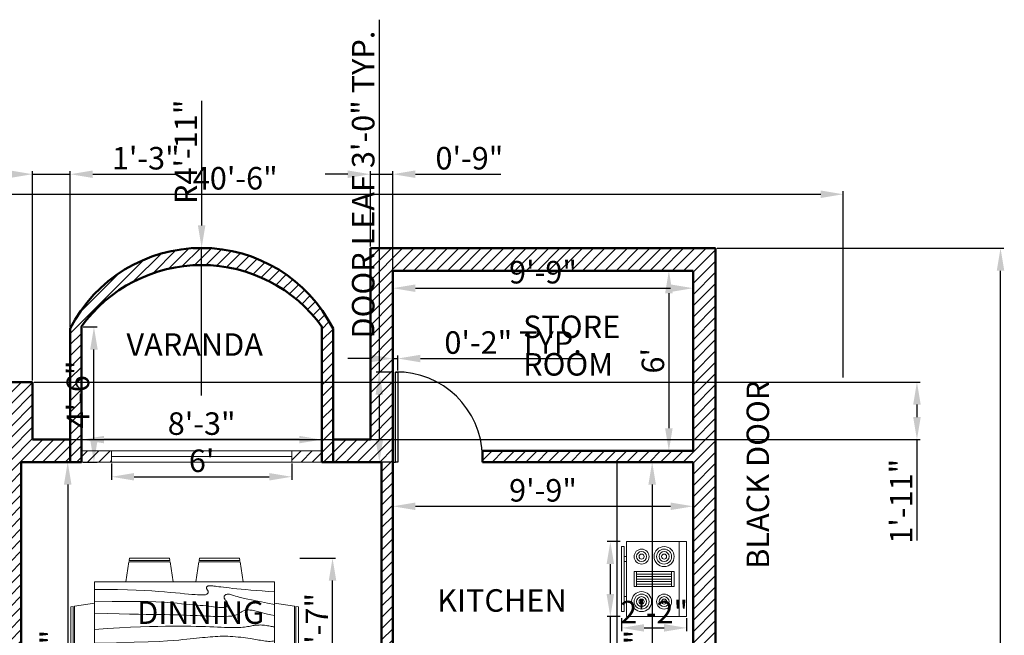
# Model space of a CAD drawing. Units: inches. Extents: x 5928 to 6612, y 5674 to 6320.
# Tile 5 of 5: x 6219 to 6612, y 6074 to 6320. Entities that reach past the tile are written whole.
import ezdxf

# ---------------------------------------------------------------- set-up
doc = ezdxf.new("R2010")
doc.units = ezdxf.units.IN
for name, color, linetype, lineweight in [('A-ANNO-DIMS', 2, 'Continuous', 18), ('A-ANNO-TEXT', 7, 'Continuous', 25), ('A-AREA-IDEN', 7, 'Continuous', 25), ('A-DOOR', 3, 'Continuous', 25), ('A-EQPM', 9, 'Continuous', 18), ('A-FLOR-CASE', 8, 'Continuous', 25), ('A-FURN', 8, 'Continuous', 18), ('A-GLAZ', 4, 'Continuous', 18), ('A-WALL', 7, 'Continuous', 50), ('A-WALL-PATT', 252, 'Continuous', 13)]:
    doc.layers.add(name, color=color, linetype=linetype, lineweight=lineweight)
doc.styles.get("Standard").update_dxf_attribs({"font": 'arial.ttf'})
doc.dimstyles.new('ISO-25', dxfattribs={"dimtxt": 9, "dimasz": 9, "dimexe": 1.25, "dimexo": 0.625, "dimtad": 1, "dimdec": 1, "dimrnd": 9, "dimlunit": 3, "dimtxsty": 'Standard', "dimcen": 2.5, "dimadec": 0, "dimazin": 0, "dimtfac": 1, "dimtdec": 1, "dimtmove": 0, "dimatfit": 3, "dimfxl": 1, "dimarcsym": 0})

# ---------------------------------------------------------------- blocks, each defined once
blk = doc.blocks.new('Dining Set - 36 x 72 in.')
for p, q in [((-22.2343, 26.00059), (-23.4847, 17.99762)), ((-22.2304, 26), (-5.7608, 26)), ((-22, 27.5), (-22.1562, 26.50042)), ((-5.8416, 26.5), (-22.1534, 26.5)), ((-22, 27.5), (-6, 27.5)), ((-5.8437, 26.49966), (-6, 27.5)), ((-4.5152, 17.99762), (-5.7655, 25.99926)), ((5.7657, 26.00059), (4.5153, 17.99762)), ((5.7696, 26), (22.2392, 26)), ((6, 27.5), (5.8438, 26.50042)), ((22.1584, 26.5), (5.8466, 26.5)), ((6, 27.5), (22, 27.5)), ((22.1563, 26.49966), (22, 27.5)), ((23.4848, 17.99762), (22.2345, 25.99926)), ((36, 18), (-36, 18)), ((-36, 18), (-36, -18)), ((36, -18), (36, 18)), ((-45.5, 8), (-44.5004, 8.15617)), ((-45.5, 8), (-45.5, -8)), ((-44.5, -8.15843), (-44.5, 8.15338)), ((-44.0006, 8.23428), (-35.9976, 9.48474)), ((-44, 8.23041), (-44, -8.23915)), ((44.0006, 8.23428), (35.9976, 9.48474)), ((44, 8.23041), (44, -8.23915)), ((44.5, -8.15843), (44.5, 8.15338)), ((45.5, 8), (44.5005, 8.15617)), ((45.5, 8), (45.5, -8)), ((-44.4997, -8.15631), (-45.5, -8)), ((-35.9976, -9.48476), (-43.9993, -8.2345)), ((35.9976, -9.48476), (43.9993, -8.2345)), ((44.4997, -8.15631), (45.5, -8)), ((-36, -18), (36, -18)), ((-22.2343, -26.0006), (-23.4847, -17.99762)), ((-4.5152, -17.99762), (-5.7655, -25.99928)), ((5.7657, -26.0006), (4.5153, -17.99762)), ((23.4848, -17.99762), (22.2345, -25.99928)), ((-22.2304, -26), (-5.7608, -26)), ((-22, -27.5), (-22.1562, -26.50044)), ((-5.8416, -26.5), (-22.1534, -26.5)), ((-22, -27.5), (-6, -27.5)), ((-5.8437, -26.49967), (-6, -27.5)), ((5.7696, -26), (22.2392, -26)), ((6, -27.5), (5.8438, -26.50044)), ((22.1584, -26.5), (5.8466, -26.5)), ((6, -27.5), (22, -27.5)), ((22.1563, -26.49967), (22, -27.5))]:
    blk.add_line(p, q)
for points in [[(-36, 15), (-31.1772, 14.97754), (-26.8079, 14.91406), (-22.8538, 14.81543), (-19.276, 14.6875), (-16.0362, 14.53613), (-13.0957, 14.36718), (-10.4159, 14.18652), (-7.9583, 14), (-5.6904, 13.81315), (-3.6035, 13.63021), (-1.6954, 13.45508), (0.0365, 13.29166), (1.5945, 13.14388), (2.9811, 13.01562), (4.1988, 12.9108), (5.25, 12.83333), (6.1393, 12.78613), (6.8802, 12.76823), (7.4883, 12.77767), (7.9792, 12.8125), (8.3685, 12.87077), (8.6719, 12.95052), (8.9049, 13.0498), (9.0833, 13.16666), (9.2205, 13.29899), (9.3216, 13.44401), (9.3895, 13.59879), (9.4271, 13.76041), (9.4373, 13.92594), (9.4232, 14.09245), (9.3875, 14.257), (9.3333, 14.41666), (9.2638, 14.56917), (9.1836, 14.71484), (9.0975, 14.85465), (9.0104, 14.98958), (8.9272, 15.1206), (8.8529, 15.2487), (8.7922, 15.37483), (8.75, 15.5), (8.7305, 15.62467), (8.7344, 15.74739), (8.7617, 15.86621), (8.8125, 15.97916), (8.8867, 16.08431), (8.9844, 16.17968), (9.1055, 16.26334), (9.25, 16.33333), (9.4189, 16.38802), (9.6172, 16.42708), (9.8506, 16.45052), (10.125, 16.45833), (10.4463, 16.45052), (10.8203, 16.42708), (11.2529, 16.38802), (11.75, 16.33333), (12.3184, 16.26318), (12.9694, 16.17838), (13.7151, 16.07991), (14.5677, 15.96875), (15.5395, 15.84586), (16.6426, 15.71224), (17.8893, 15.56884), (19.2917, 15.41666), (20.859, 15.25667), (22.5879, 15.08984), (24.4721, 14.91715), (26.5052, 14.73958), (28.6809, 14.5581), (30.9929, 14.3737), (33.4347, 14.18733), (36, 14)], [(-36, 10), (-28.9766, 10.14274), (-23.1725, 10.20442), (-18.4241, 10.19775), (-14.5677, 10.13541), (-11.4399, 10.03011), (-8.877, 9.89453), (-6.7154, 9.74137), (-4.7917, 9.58333), (-2.9698, 9.43082), (-1.2246, 9.28515), (0.4415, 9.14534), (2.026, 9.01041), (3.5266, 8.87939), (4.9408, 8.7513), (6.266, 8.62516), (7.5, 8.5), (8.6411, 8.37549), (9.6914, 8.2539), (10.6538, 8.13818), (11.5312, 8.03125), (12.3267, 7.93603), (13.043, 7.85547), (13.6831, 7.79248), (14.25, 7.75), (14.7471, 7.7303), (15.1797, 7.73307), (15.5537, 7.75732), (15.875, 7.80208), (16.1494, 7.86637), (16.3828, 7.94922), (16.5811, 8.04964), (16.75, 8.16666), (16.8944, 8.29915), (17.0143, 8.44531), (17.1089, 8.60319), (17.1771, 8.77083), (17.218, 8.94629), (17.2305, 9.1276), (17.2137, 9.31282), (17.1667, 9.5), (17.0895, 9.6875), (16.987, 9.875), (16.8649, 10.0625), (16.7292, 10.25), (16.5856, 10.4375), (16.4401, 10.625), (16.2985, 10.8125), (16.1667, 11), (16.05, 11.18733), (15.9518, 11.3737), (15.8752, 11.5581), (15.8229, 11.73958), (15.798, 11.91715), (15.8034, 12.08984), (15.842, 12.25667), (15.9167, 12.41666), (16.0295, 12.56836), (16.1784, 12.70833), (16.3605, 12.83268), (16.5729, 12.9375), (16.8127, 13.01888), (17.0768, 13.07291), (17.3625, 13.0957), (17.6667, 13.08333), (17.9894, 13.03312), (18.3418, 12.94726), (18.7382, 12.82918), (19.1927, 12.68229), (19.7195, 12.51001), (20.3327, 12.31575), (21.0465, 12.10294), (21.875, 11.875), (22.8357, 11.63354), (23.959, 11.37304), (25.2786, 11.08618), (26.8282, 10.76562), (28.6414, 10.40405), (30.752, 9.99414), (33.1936, 9.52856), (36, 9)], [(-36, 5.5), (-30.7157, 5.3348), (-26.069, 5.20963), (-21.9946, 5.11767), (-18.4271, 5.05208), (-15.3009, 5.00602), (-12.5508, 4.97265), (-10.1112, 4.94515), (-7.9167, 4.91666), (-5.909, 4.88167), (-4.0586, 4.83984), (-2.3429, 4.79215), (-0.7396, 4.73958), (0.7739, 4.6831), (2.22, 4.6237), (3.6213, 4.56233), (5, 4.5), (6.373, 4.43782), (7.7344, 4.3776), (9.0723, 4.32129), (10.375, 4.27083), (11.6309, 4.22819), (12.8281, 4.19531), (13.9551, 4.17415), (15, 4.16666), (15.954, 4.17448), (16.819, 4.19791), (17.6001, 4.23698), (18.3021, 4.29166), (18.9299, 4.36198), (19.4883, 4.44791), (19.9823, 4.54948), (20.4167, 4.66666), (20.7969, 4.79899), (21.1302, 4.94401), (21.4245, 5.09879), (21.6875, 5.26041), (21.9271, 5.42594), (22.1511, 5.59245), (22.3672, 5.757), (22.5834, 5.91666), (22.8065, 6.06868), (23.0404, 6.21093), (23.2879, 6.34147), (23.5521, 6.45833), (23.8358, 6.55957), (24.142, 6.64323), (24.4735, 6.70735), (24.8334, 6.75), (25.2235, 6.76969), (25.642, 6.76692), (26.0858, 6.74267), (26.5521, 6.69791), (27.0379, 6.63362), (27.5404, 6.55078), (28.0565, 6.45036), (28.5834, 6.33333), (29.1242, 6.19987), (29.7071, 6.04687), (30.3661, 5.87044), (31.1354, 5.66666), (32.0493, 5.43164), (33.142, 5.16146), (34.4475, 4.85221), (36, 4.5)], [(-36, -1), (-30.7915, -0.6591), (-26.0195, -0.38216), (-21.6519, -0.16284), (-17.6563, 0.00521), (-14.0005, 0.12833), (-10.6523, 0.21289), (-7.5796, 0.26522), (-4.75, 0.29166), (-2.134, 0.29793), (0.2878, 0.28711), (2.5317, 0.26163), (4.6146, 0.22396), (6.5529, 0.17651), (8.3633, 0.12174), (10.0623, 0.06209), (11.6667, 0), (13.1899, -0.06201), (14.6341, -0.1211), (15.9982, -0.17432), (17.2813, -0.21875), (18.4823, -0.25147), (19.6003, -0.26953), (20.6343, -0.27002), (21.5834, -0.25), (22.4481, -0.20768), (23.2357, -0.14584), (23.9549, -0.06836), (24.6146, 0.02083), (25.2235, 0.11784), (25.7904, 0.21875), (26.3241, 0.31966), (26.8334, 0.41666), (27.3265, 0.50618), (27.8099, 0.58593), (28.2894, 0.65397), (28.7709, 0.70833), (29.2601, 0.74707), (29.763, 0.76823), (30.2855, 0.76985), (30.8334, 0.75), (31.4088, 0.70784), (31.9994, 0.64713), (32.589, 0.57275), (33.1615, 0.48958), (33.7008, 0.4025), (34.1908, 0.3164), (34.6153, 0.23616), (34.9584, 0.16666), (35.2099, 0.11165), (35.3848, 0.07031), (35.504, 0.04069), (35.5886, 0.02083), (35.6594, 0.00879), (35.7377, 0.0026), (35.8442, 0.00032), (36, 0)], [(-36, -6.5), (-27.1843, -6.31267), (-20.084, -6.1263), (-14.469, -5.9419), (-10.1094, -5.76042), (-6.7752, -5.58285), (-4.2363, -5.41016), (-2.2629, -5.24333), (-0.625, -5.08334), (0.8708, -4.93099), (2.2715, -4.78646), (3.5872, -4.64974), (4.8281, -4.52084), (6.0046, -4.39974), (7.127, -4.28646), (8.2053, -4.18099), (9.25, -4.08334), (10.2705, -3.99382), (11.2734, -3.91407), (12.2647, -3.84603), (13.25, -3.79167), (14.2354, -3.75293), (15.2266, -3.73177), (16.2295, -3.73015), (17.25, -3.75), (18.2912, -3.79248), (19.3451, -3.85547), (20.4009, -3.93604), (21.4479, -4.03125), (22.4754, -4.13819), (23.4727, -4.25391), (24.4289, -4.37549), (25.3334, -4.5), (26.1785, -4.62492), (26.9694, -4.74935), (27.7145, -4.87281), (28.4219, -4.99479), (29.1, -5.11483), (29.7572, -5.23242), (30.4016, -5.34709), (31.0417, -5.45834), (31.6837, -5.56437), (32.3262, -5.65821), (32.9658, -5.73153), (33.599, -5.77604), (34.2224, -5.78345), (34.8327, -5.74545), (35.4264, -5.65373), (36, -5.5)], [(-36, -10), (-26.4022, -9.81299), (-18.4675, -9.62891), (-11.9839, -9.45069), (-6.7396, -9.28125), (-2.5226, -9.12354), (0.8789, -8.98047), (3.6769, -8.85498), (6.0833, -8.75), (8.2767, -8.66765), (10.3021, -8.60677), (12.1712, -8.56543), (13.8958, -8.54167), (15.4876, -8.53353), (16.9583, -8.53907), (18.3197, -8.55632), (19.5834, -8.58334), (20.7616, -8.61841), (21.8685, -8.66081), (22.9188, -8.71004), (23.9271, -8.76563), (24.9081, -8.82707), (25.8763, -8.89388), (26.8465, -8.96558), (27.8334, -9.04167), (28.8474, -9.12118), (29.8828, -9.20117), (30.93, -9.27824), (31.9792, -9.34896), (33.0205, -9.40991), (34.0443, -9.45768), (35.0407, -9.48885), (36, -9.5)], [(-36, -14.5), (-30.0881, -14.33513), (-25.0332, -14.21224), (-20.7312, -14.12647), (-17.0781, -14.07292), (-13.97, -14.04671), (-11.3027, -14.04297), (-8.9724, -14.05681), (-6.875, -14.08334), (-4.9224, -14.11833), (-3.0905, -14.16016), (-1.3709, -14.20785), (0.2448, -14.26042), (1.7647, -14.3169), (3.1973, -14.3763), (4.5507, -14.43767), (5.8333, -14.5), (7.0554, -14.5621), (8.235, -14.62175), (9.3922, -14.67652), (10.5469, -14.72396), (11.7192, -14.76164), (12.929, -14.78711), (14.1965, -14.79794), (15.5417, -14.79167), (16.9933, -14.76424), (18.6152, -14.70508), (20.4804, -14.60197), (22.6615, -14.44271), (25.2312, -14.21509), (28.2624, -13.9069), (31.8277, -13.50594), (36, -13)]]:
    blk.add_lwpolyline(points)
blk = doc.blocks.new('Range-Oven - 30 in top')
for p, q in [((0, -3), (30, -3)), ((12, -6), (18, -6)), ((13, -20), (13, -6)), ((14, -6), (14, -20)), ((15, -20), (15, -6)), ((16, -6), (16, -20)), ((17, -20), (17, -6)), ((18, -20), (12, -20)), ((6, -24), (6, -25)), ((8, -25), (8, -24)), ((22, -25), (22, -24)), ((24, -24), (24, -25))]:
    blk.add_line(p, q)
for points in [[(0, -24), (0, 0), (30, 0), (30, -24)], [(12, -21), (12, -5), (18, -5), (18, -21)], [(2, -26), (2, -25), (28, -25), (28, -26)]]:
    blk.add_lwpolyline(points, close=True)
for centre, radius in [((6, -9), 4), ((6, -9), 3), ((6, -9), 2), ((24, -9), 3), ((24, -9), 2), ((6, -9), 1), ((24, -9), 1), ((6, -18), 3), ((24, -18), 4), ((24, -18), 3), ((6, -18), 2), ((6, -18), 1), ((24, -18), 2), ((24, -18), 1)]:
    blk.add_circle(centre, radius)
blk = doc.blocks.new('*D23')
at = {"layer": 'A-ANNO-DIMS', "color": 0, "lineweight": -2, "transparency": 16777216}
for p, q in [((6220.15, 6142.76), (6239.34, 6142.76)), ((6238.09, 6133.76), (6238.09, 5983.76)), ((6220.15, 5974.76), (6239.34, 5974.76))]:
    blk.add_line(p, q, dxfattribs=at)
at = {"layer": 'A-ANNO-DIMS', "color": 0, "transparency": 16777216}
for points in [[(6236.59, 6133.76), (6239.59, 6133.76), (6238.09, 6142.76)], [(6236.59, 5983.76), (6239.59, 5983.76), (6238.09, 5974.76)]]:
    blk.add_solid(points, dxfattribs=at)
at = {"layer": 'Defpoints', "color": 0, "transparency": 16777216}
for p in [(6219.53, 6142.76), (6219.53, 5974.76), (6238.09, 5974.76)]:
    blk.add_point(p, dxfattribs=at)
at = {"layer": 'A-ANNO-DIMS', "color": 0, "transparency": 16777216, "insert": (6232.87, 6058.76), "char_height": 9, "attachment_point": 5, "rotation": 90}
blk.add_mtext('14\'-3"', dxfattribs=at)
blk = doc.blocks.new('*D27')
at = {"layer": 'A-ANNO-DIMS', "color": 0, "lineweight": -2, "transparency": 16777216}
for p, q in [((6243.61, 6147.89), (6243.61, 6153)), ((6330.61, 6151.75), (6252.61, 6151.75)), ((6339.61, 6147.89), (6339.61, 6153))]:
    blk.add_line(p, q, dxfattribs=at)
at = {"layer": 'A-ANNO-DIMS', "color": 0, "transparency": 16777216}
for points in [[(6252.61, 6153.25), (6252.61, 6150.25), (6243.61, 6151.75)], [(6330.61, 6153.25), (6330.61, 6150.25), (6339.61, 6151.75)]]:
    blk.add_solid(points, dxfattribs=at)
at = {"layer": 'Defpoints', "color": 0, "transparency": 16777216}
for p in [(6243.61, 6151.75), (6243.61, 6147.26), (6339.61, 6147.26)]:
    blk.add_point(p, dxfattribs=at)
at = {"layer": 'A-ANNO-DIMS', "color": 0, "transparency": 16777216, "insert": (6291.61, 6156.98), "char_height": 9, "attachment_point": 5}
blk.add_mtext('8\'-3"', dxfattribs=at)
blk = doc.blocks.new('*D28')
at = {"layer": 'A-ANNO-DIMS', "color": 0, "lineweight": -2, "transparency": 16777216}
for p, q in [((6255.61, 6142.14), (6255.61, 6135.65)), ((6327.61, 6142.14), (6327.61, 6135.65)), ((6264.61, 6136.9), (6318.61, 6136.9))]:
    blk.add_line(p, q, dxfattribs=at)
at = {"layer": 'A-ANNO-DIMS', "color": 0, "transparency": 16777216}
for points in [[(6264.61, 6138.4), (6264.61, 6135.4), (6255.61, 6136.9)], [(6318.61, 6138.4), (6318.61, 6135.4), (6327.61, 6136.9)]]:
    blk.add_solid(points, dxfattribs=at)
at = {"layer": 'Defpoints', "color": 0, "transparency": 16777216}
for p in [(6255.61, 6142.76), (6327.61, 6142.76), (6327.61, 6136.9)]:
    blk.add_point(p, dxfattribs=at)
at = {"layer": 'A-ANNO-DIMS', "color": 0, "transparency": 16777216, "insert": (6291.61, 6142.12), "char_height": 9, "attachment_point": 5}
blk.add_mtext("6'", dxfattribs=at)
blk = doc.blocks.new('*D29')
at = {"layer": 'A-ANNO-DIMS', "color": 0, "lineweight": -2, "transparency": 16777216}
for p, q in [((6244.23, 6196.76), (6249.81, 6196.76)), ((6248.56, 6151.76), (6248.56, 6187.76)), ((6244.23, 6142.76), (6249.81, 6142.76))]:
    blk.add_line(p, q, dxfattribs=at)
at = {"layer": 'A-ANNO-DIMS', "color": 0, "transparency": 16777216}
for points in [[(6247.06, 6187.76), (6250.06, 6187.76), (6248.56, 6196.76)], [(6247.06, 6151.76), (6250.06, 6151.76), (6248.56, 6142.76)]]:
    blk.add_solid(points, dxfattribs=at)
at = {"layer": 'Defpoints', "color": 0, "transparency": 16777216}
for p in [(6243.61, 6196.76), (6248.56, 6196.76), (6243.61, 6142.76)]:
    blk.add_point(p, dxfattribs=at)
at = {"layer": 'A-ANNO-DIMS', "color": 0, "transparency": 16777216, "insert": (6243.34, 6169.76), "char_height": 9, "attachment_point": 5, "rotation": 90}
blk.add_mtext('4\'-6"', dxfattribs=at)
blk = doc.blocks.new('*D30')
at = {"layer": 'A-ANNO-DIMS', "color": 0, "lineweight": -2, "transparency": 16777216}
for p, q in [((6368.03, 6218.64), (6368.03, 6211.02)), ((6488.03, 6218.64), (6488.03, 6211.02)), ((6377.03, 6212.27), (6479.03, 6212.27))]:
    blk.add_line(p, q, dxfattribs=at)
at = {"layer": 'A-ANNO-DIMS', "color": 0, "transparency": 16777216}
for points in [[(6377.03, 6213.77), (6377.03, 6210.77), (6368.03, 6212.27)], [(6479.03, 6213.77), (6479.03, 6210.77), (6488.03, 6212.27)]]:
    blk.add_solid(points, dxfattribs=at)
at = {"layer": 'Defpoints', "color": 0, "transparency": 16777216}
for p in [(6368.03, 6219.26), (6488.03, 6219.26), (6488.03, 6212.27)]:
    blk.add_point(p, dxfattribs=at)
at = {"layer": 'A-ANNO-DIMS', "color": 0, "transparency": 16777216, "insert": (6428.03, 6217.49), "char_height": 9, "attachment_point": 5}
blk.add_mtext('9\'-9"', dxfattribs=at)
blk = doc.blocks.new('*D31')
at = {"layer": 'A-ANNO-DIMS', "color": 0, "lineweight": -2, "transparency": 16777216}
for p, q in [((6487.4, 6219.26), (6477.09, 6219.26)), ((6478.34, 6210.26), (6478.34, 6156.26)), ((6487.4, 6147.26), (6477.09, 6147.26))]:
    blk.add_line(p, q, dxfattribs=at)
at = {"layer": 'A-ANNO-DIMS', "color": 0, "transparency": 16777216}
for points in [[(6476.84, 6210.26), (6479.84, 6210.26), (6478.34, 6219.26)], [(6476.84, 6156.26), (6479.84, 6156.26), (6478.34, 6147.26)]]:
    blk.add_solid(points, dxfattribs=at)
at = {"layer": 'Defpoints', "color": 0, "transparency": 16777216}
for p in [(6488.03, 6219.26), (6478.34, 6147.26), (6488.03, 6147.26)]:
    blk.add_point(p, dxfattribs=at)
at = {"layer": 'A-ANNO-DIMS', "color": 0, "transparency": 16777216, "insert": (6473.12, 6183.26), "char_height": 9, "attachment_point": 5, "rotation": 90}
blk.add_mtext("6'", dxfattribs=at)
blk = doc.blocks.new('*D34')
at = {"layer": 'A-ANNO-DIMS', "color": 0, "lineweight": -2, "transparency": 16777216}
for p, q in [((6487.4, 6142.76), (6470.41, 6142.76)), ((6471.66, 6133.76), (6471.66, 5983.76)), ((6487.4, 5974.76), (6470.41, 5974.76))]:
    blk.add_line(p, q, dxfattribs=at)
at = {"layer": 'A-ANNO-DIMS', "color": 0, "transparency": 16777216}
for points in [[(6470.16, 6133.76), (6473.16, 6133.76), (6471.66, 6142.76)], [(6470.16, 5983.76), (6473.16, 5983.76), (6471.66, 5974.76)]]:
    blk.add_solid(points, dxfattribs=at)
at = {"layer": 'Defpoints', "color": 0, "transparency": 16777216}
for p in [(6488.03, 6142.76), (6471.66, 5974.76), (6488.03, 5974.76)]:
    blk.add_point(p, dxfattribs=at)
at = {"layer": 'A-ANNO-DIMS', "color": 0, "transparency": 16777216, "insert": (6466.44, 6058.76), "char_height": 9, "attachment_point": 5, "rotation": 90}
blk.add_mtext('14\'-3"', dxfattribs=at)
blk = doc.blocks.new('*D35')
at = {"layer": 'A-ANNO-DIMS', "color": 0, "lineweight": -2, "transparency": 16777216}
for p, q in [((6368.03, 6142.14), (6368.03, 6123.85)), ((6488.03, 6142.14), (6488.03, 6123.85)), ((6377.03, 6125.1), (6479.03, 6125.1))]:
    blk.add_line(p, q, dxfattribs=at)
at = {"layer": 'A-ANNO-DIMS', "color": 0, "transparency": 16777216}
for points in [[(6377.03, 6126.6), (6377.03, 6123.6), (6368.03, 6125.1)], [(6479.03, 6126.6), (6479.03, 6123.6), (6488.03, 6125.1)]]:
    blk.add_solid(points, dxfattribs=at)
at = {"layer": 'Defpoints', "color": 0, "transparency": 16777216}
for p in [(6368.03, 6142.76), (6488.03, 6142.76), (6488.03, 6125.1)]:
    blk.add_point(p, dxfattribs=at)
at = {"layer": 'A-ANNO-DIMS', "color": 0, "transparency": 16777216, "insert": (6428.03, 6130.32), "char_height": 9, "attachment_point": 5}
blk.add_mtext('9\'-9"', dxfattribs=at)
blk = doc.blocks.new('*D36')
at = {"layer": 'A-ANNO-DIMS', "color": 0, "lineweight": -2, "transparency": 16777216}
for p, q in [((6062.03, 6175.39), (6062.03, 6251.06)), ((6071.03, 6249.81), (6539.03, 6249.81)), ((6548.03, 6176.51), (6548.03, 6251.06))]:
    blk.add_line(p, q, dxfattribs=at)
at = {"layer": 'A-ANNO-DIMS', "color": 0, "transparency": 16777216}
for points in [[(6071.03, 6251.31), (6071.03, 6248.31), (6062.03, 6249.81)], [(6539.03, 6251.31), (6539.03, 6248.31), (6548.03, 6249.81)]]:
    blk.add_solid(points, dxfattribs=at)
at = {"layer": 'Defpoints', "color": 0, "transparency": 16777216}
for p in [(6548.03, 6249.81), (6062.03, 6174.76), (6548.03, 6175.89)]:
    blk.add_point(p, dxfattribs=at)
at = {"layer": 'A-ANNO-DIMS', "color": 0, "transparency": 16777216, "insert": (6305.03, 6255.03), "char_height": 9, "attachment_point": 5}
blk.add_mtext('40\'-6"', dxfattribs=at)
blk = doc.blocks.new('*D37')
at = {"layer": 'A-ANNO-DIMS', "color": 0, "lineweight": -2, "transparency": 16777216}
for p, q in [((6497.65, 6228.26), (6612.14, 6228.26)), ((6610.89, 5720.26), (6610.89, 6219.26)), ((6424.38, 5711.26), (6612.14, 5711.26))]:
    blk.add_line(p, q, dxfattribs=at)
at = {"layer": 'A-ANNO-DIMS', "color": 0, "transparency": 16777216}
for points in [[(6609.39, 6219.26), (6612.39, 6219.26), (6610.89, 6228.26)], [(6609.39, 5720.26), (6612.39, 5720.26), (6610.89, 5711.26)]]:
    blk.add_solid(points, dxfattribs=at)
at = {"layer": 'Defpoints', "color": 0, "transparency": 16777216}
for p in [(6497.03, 6228.26), (6610.89, 6228.26), (6423.76, 5711.26)]:
    blk.add_point(p, dxfattribs=at)
at = {"layer": 'A-ANNO-DIMS', "color": 0, "transparency": 16777216, "insert": (6605.67, 5969.76), "char_height": 9, "attachment_point": 5, "rotation": 90}
blk.add_mtext('42\'-9"', dxfattribs=at)
blk = doc.blocks.new('DOOR-LEAF-36IN')
for p, q in [((0, 0), (0, 36)), ((0, 36), (1, 36)), ((1, 36), (1, 0)), ((-1, 0), (0, 0)), ((1, 0), (0, 0))]:
    blk.add_line(p, q)
blk = doc.blocks.new('*D58')
at = {"layer": 'A-ANNO-DIMS', "color": 0, "lineweight": -2, "transparency": 16777216}
for p, q in [((6362.63, 6178.76), (6362.63, 6319.58)), ((6367.4, 6178.76), (6361.38, 6178.76)), ((6362.63, 6151.76), (6362.63, 6169.76)), ((6367.4, 6142.76), (6361.38, 6142.76))]:
    blk.add_line(p, q, dxfattribs=at)
at = {"layer": 'A-ANNO-DIMS', "color": 0, "transparency": 16777216}
for points in [[(6361.13, 6169.76), (6364.13, 6169.76), (6362.63, 6178.76)], [(6361.13, 6151.76), (6364.13, 6151.76), (6362.63, 6142.76)]]:
    blk.add_solid(points, dxfattribs=at)
at = {"layer": 'Defpoints', "color": 0, "transparency": 16777216}
for p in [(6362.63, 6178.76), (6368.03, 6178.76), (6368.03, 6142.76)]:
    blk.add_point(p, dxfattribs=at)
at = {"layer": 'A-ANNO-DIMS', "color": 0, "transparency": 16777216, "insert": (6357.34, 6253.67), "char_height": 9, "attachment_point": 5, "rotation": 90}
blk.add_mtext('DOOR LEAF 3\'-0" TYP.', dxfattribs=at)
blk = doc.blocks.new('*D59')
at = {"layer": 'A-ANNO-DIMS', "color": 0, "lineweight": -2, "transparency": 16777216}
for p, q in [((6359.03, 6184.16), (6350.03, 6184.16)), ((6368.03, 6179.39), (6368.03, 6185.41)), ((6368.03, 6184.16), (6370.03, 6184.16)), ((6370.03, 6179.39), (6370.03, 6185.41)), ((6379.03, 6184.16), (6444.14, 6184.16))]:
    blk.add_line(p, q, dxfattribs=at)
at = {"layer": 'A-ANNO-DIMS', "color": 0, "transparency": 16777216}
for points in [[(6359.03, 6185.66), (6359.03, 6182.66), (6368.03, 6184.16)], [(6379.03, 6185.66), (6379.03, 6182.66), (6370.03, 6184.16)]]:
    blk.add_solid(points, dxfattribs=at)
at = {"layer": 'Defpoints', "color": 0, "transparency": 16777216}
for p in [(6370.03, 6184.16), (6368.03, 6178.76), (6370.03, 6178.76)]:
    blk.add_point(p, dxfattribs=at)
at = {"layer": 'A-ANNO-DIMS', "color": 0, "transparency": 16777216, "insert": (6416.08, 6189.38), "char_height": 9, "attachment_point": 5}
blk.add_mtext('0\'-2" TYP.', dxfattribs=at)
blk = doc.blocks.new('*D65')
at = {"layer": 'A-ANNO-DIMS', "color": 0, "lineweight": -2, "transparency": 16777216}
for p, q in [((6330.9, 6104.39), (6345.17, 6104.39)), ((6343.92, 6058.39), (6343.92, 6095.39)), ((6330.9, 6049.39), (6345.17, 6049.39))]:
    blk.add_line(p, q, dxfattribs=at)
at = {"layer": 'A-ANNO-DIMS', "color": 0, "transparency": 16777216}
for points in [[(6342.42, 6095.39), (6345.42, 6095.39), (6343.92, 6104.39)], [(6342.42, 6058.39), (6345.42, 6058.39), (6343.92, 6049.39)]]:
    blk.add_solid(points, dxfattribs=at)
at = {"layer": 'Defpoints', "color": 0, "transparency": 16777216}
for p in [(6330.27, 6104.39), (6343.92, 6104.39), (6330.27, 6049.39)]:
    blk.add_point(p, dxfattribs=at)
at = {"layer": 'A-ANNO-DIMS', "color": 0, "transparency": 16777216, "insert": (6338.8, 6076.89), "char_height": 9, "attachment_point": 5, "rotation": 90}
blk.add_mtext('4\'-7"', dxfattribs=at)
blk = doc.blocks.new('*D66')
at = {"layer": 'A-ANNO-DIMS', "color": 0, "lineweight": -2, "transparency": 16777216}
for p, q in [((6458.82, 6111), (6453.69, 6111)), ((6454.94, 6102), (6454.94, 6090)), ((6458.82, 6081), (6453.69, 6081)), ((6454.94, 6081), (6454.94, 5999.09))]:
    blk.add_line(p, q, dxfattribs=at)
at = {"layer": 'A-ANNO-DIMS', "color": 0, "transparency": 16777216}
for points in [[(6453.44, 6102), (6456.44, 6102), (6454.94, 6111)], [(6453.44, 6090), (6456.44, 6090), (6454.94, 6081)]]:
    blk.add_solid(points, dxfattribs=at)
at = {"layer": 'Defpoints', "color": 0, "transparency": 16777216}
for p in [(6459.44, 6111), (6454.94, 6081), (6459.44, 6081)]:
    blk.add_point(p, dxfattribs=at)
at = {"layer": 'A-ANNO-DIMS', "color": 0, "transparency": 16777216, "insert": (6449.67, 6035.54), "char_height": 9, "attachment_point": 5, "rotation": 90}
blk.add_mtext('RANGE 2\'-6"', dxfattribs=at)
blk = doc.blocks.new('*D67')
at = {"layer": 'A-ANNO-DIMS', "color": 0, "lineweight": -2, "transparency": 16777216}
for p, q in [((6459.44, 6080.37), (6459.44, 6075.25)), ((6485.44, 6080.37), (6485.44, 6075.25)), ((6468.44, 6076.5), (6476.44, 6076.5))]:
    blk.add_line(p, q, dxfattribs=at)
at = {"layer": 'A-ANNO-DIMS', "color": 0, "transparency": 16777216}
for points in [[(6468.44, 6078), (6468.44, 6075), (6459.44, 6076.5)], [(6476.44, 6078), (6476.44, 6075), (6485.44, 6076.5)]]:
    blk.add_solid(points, dxfattribs=at)
at = {"layer": 'Defpoints', "color": 0, "transparency": 16777216}
for p in [(6459.44, 6081), (6485.44, 6081), (6485.44, 6076.5)]:
    blk.add_point(p, dxfattribs=at)
at = {"layer": 'A-ANNO-DIMS', "color": 0, "transparency": 16777216, "insert": (6472.44, 6081.64), "char_height": 9, "attachment_point": 5}
blk.add_mtext('2\'-2"', dxfattribs=at)
blk = doc.blocks.new('*D73')
at = {"layer": 'A-ANNO-DIMS', "color": 0, "lineweight": -2, "transparency": 16777216}
for p, q in [((6215.03, 6257.82), (6206.03, 6257.82)), ((6224.03, 6175.39), (6224.03, 6259.07)), ((6224.03, 6257.82), (6239.11, 6257.82)), ((6239.11, 6196.83), (6239.11, 6259.07)), ((6248.11, 6257.82), (6281.43, 6257.82))]:
    blk.add_line(p, q, dxfattribs=at)
at = {"layer": 'A-ANNO-DIMS', "color": 0, "transparency": 16777216}
for points in [[(6215.03, 6259.32), (6215.03, 6256.32), (6224.03, 6257.82)], [(6248.11, 6259.32), (6248.11, 6256.32), (6239.11, 6257.82)]]:
    blk.add_solid(points, dxfattribs=at)
at = {"layer": 'Defpoints', "color": 0, "transparency": 16777216}
for p in [(6239.11, 6257.82), (6239.11, 6196.21), (6224.03, 6174.76)]:
    blk.add_point(p, dxfattribs=at)
at = {"layer": 'A-ANNO-DIMS', "color": 0, "transparency": 16777216, "insert": (6269.27, 6263.04), "char_height": 9, "attachment_point": 5}
blk.add_mtext('1\'-3"', dxfattribs=at)
blk = doc.blocks.new('*D74')
at = {"layer": 'A-ANNO-DIMS', "color": 0, "lineweight": -2, "transparency": 16777216}
for p, q in [((6224.65, 6174.76), (6578.73, 6174.76)), ((6577.48, 6165.76), (6577.48, 6160.76)), ((6224.65, 6151.76), (6578.73, 6151.76)), ((6577.48, 6151.76), (6577.48, 6111.44))]:
    blk.add_line(p, q, dxfattribs=at)
at = {"layer": 'A-ANNO-DIMS', "color": 0, "transparency": 16777216}
for points in [[(6575.98, 6165.76), (6578.98, 6165.76), (6577.48, 6174.76)], [(6575.98, 6160.76), (6578.98, 6160.76), (6577.48, 6151.76)]]:
    blk.add_solid(points, dxfattribs=at)
at = {"layer": 'Defpoints', "color": 0, "transparency": 16777216}
for p in [(6224.03, 6174.76), (6224.03, 6151.76), (6577.48, 6151.76)]:
    blk.add_point(p, dxfattribs=at)
at = {"layer": 'A-ANNO-DIMS', "color": 0, "transparency": 16777216, "insert": (6572.33, 6127.1), "char_height": 9, "attachment_point": 5, "rotation": 90}
blk.add_mtext('1\'-11"', dxfattribs=at)
blk = doc.blocks.new('*D75')
at = {"layer": 'A-ANNO-DIMS', "color": 0, "lineweight": -2, "transparency": 16777216}
for p, q in [((6350.03, 6257.82), (6341.03, 6257.82)), ((6359.03, 6228.89), (6359.03, 6259.07)), ((6359.03, 6257.82), (6368.03, 6257.82)), ((6368.03, 6219.89), (6368.03, 6259.07)), ((6377.03, 6257.82), (6411.2, 6257.82))]:
    blk.add_line(p, q, dxfattribs=at)
at = {"layer": 'A-ANNO-DIMS', "color": 0, "transparency": 16777216}
for points in [[(6350.03, 6259.32), (6350.03, 6256.32), (6359.03, 6257.82)], [(6377.03, 6259.32), (6377.03, 6256.32), (6368.03, 6257.82)]]:
    blk.add_solid(points, dxfattribs=at)
at = {"layer": 'Defpoints', "color": 0, "transparency": 16777216}
for p in [(6368.03, 6257.82), (6359.03, 6228.26), (6368.03, 6219.26)]:
    blk.add_point(p, dxfattribs=at)
at = {"layer": 'A-ANNO-DIMS', "color": 0, "transparency": 16777216, "insert": (6398.61, 6263.04), "char_height": 9, "attachment_point": 5}
blk.add_mtext('0\'-9"', dxfattribs=at)
blk = doc.blocks.new('*D80')
at = {"layer": 'A-ANNO-DIMS', "color": 0, "lineweight": -2, "transparency": 16777216}
for p, q in [((6291.61, 6287.15), (6291.61, 6237.37)), ((6291.61, 6169.44), (6291.61, 6228.37))]:
    blk.add_line(p, q, dxfattribs=at)
at = {"layer": 'A-ANNO-DIMS', "color": 0, "transparency": 16777216}
blk.add_solid([(6290.11, 6237.37), (6293.11, 6237.37), (6291.61, 6228.37)], dxfattribs=at)
at = {"layer": 'Defpoints', "color": 0, "transparency": 16777216}
for p in [(6291.61, 6228.37), (6291.61, 6169.44)]:
    blk.add_point(p, dxfattribs=at)
at = {"layer": 'A-ANNO-DIMS', "color": 0, "transparency": 16777216, "insert": (6286.46, 6266.76), "char_height": 9, "attachment_point": 5, "rotation": 89.9997}
blk.add_mtext('R4\'-11"', dxfattribs=at)

msp = doc.modelspace()

# ---------------------------------------------------------------- hatches: boundary and pattern name
at = {"layer": 'A-WALL-PATT'}
h = msp.add_hatch(dxfattribs=at)
h.set_pattern_fill('ANSI31', color=256)
h.paths.add_polyline_path([(6071.03, 6165.76), (6215.03, 6165.76), (6215.03, 5969.77), (6215.03, 5950.32), (6219.53, 5950.32), (6219.53, 6142.76), (6239.11, 6142.76), (6239.11, 6151.76), (6224.03, 6151.76), (6224.03, 6174.76), (6062.03, 6174.76), (6062.03, 5969.76), (6062.03, 5894.26), (6108.76, 5894.26), (6108.76, 5711.26), (6423.76, 5711.26), (6423.76, 5750.35), (6414.76, 5750.35), (6414.76, 5720.26), (6266.26, 5720.26), (6266.26, 5862.26), (6361.1, 5862.26), (6361.1, 5866.76), (6261.76, 5866.76), (6261.76, 5720.26), (6117.76, 5720.26), (6117.76, 5792.26), (6218.26, 5792.26), (6218.26, 5796.76), (6117.76, 5796.76), (6117.76, 5898.76), (6213.76, 5898.76), (6213.76, 5828.21, -0.018207), (6216.01, 5828.09), (6218.26, 5828.09), (6218.26, 5903.26), (6117.76, 5903.26), (6071.03, 5903.26), (6071.03, 5969.77), (6071.03, 6041.26), (6117.76, 6041.26), (6172.44, 6041.26), (6172.44, 6045.76), (6117.76, 6045.76), (6071.03, 6045.76)])
h.paths.add_polyline_path([(6368.03, 6219.26), (6488.03, 6219.26), (6488.03, 6147.26), (6403.79, 6147.26), (6403.79, 6142.76), (6488.03, 6142.76), (6488.03, 5974.76), (6363.53, 5974.76), (6363.53, 5970.11), (6497.03, 5970.26), (6497.03, 6142.76), (6497.03, 6228.26), (6359.03, 6228.26), (6359.03, 6151.76), (6344.11, 6151.76), (6344.11, 6142.76), (6363.53, 6142.76), (6363.53, 6013.35), (6368.03, 6013.35), (6368.03, 6142.76)])
h.paths.add_polyline_path([(6344.11, 6196.21, 0.265753), (6295.16, 6228.26), (6288.06, 6228.26, 0.265753), (6239.11, 6196.21), (6239.11, 6142.76), (6243.61, 6142.76), (6243.61, 6196.76), (6243.45, 6196.76, -0.514089), (6339.79, 6196.74), (6339.61, 6196.76), (6339.61, 6142.76), (6344.11, 6142.76)])
h.paths.add_polyline_path([(6339.61, 6147.26), (6327.61, 6147.26), (6327.61, 6142.76), (6339.61, 6142.76)], flags=17)
h.paths.add_polyline_path([(6255.61, 6147.26), (6243.61, 6147.26), (6243.61, 6142.76), (6255.61, 6142.76)], flags=17)
h.paths.add_polyline_path([(6548.03, 5974.76), (6539.03, 5974.76), (6539.03, 5862.26), (6407.03, 5862.26), (6407.03, 5853.26), (6414.76, 5853.26), (6414.76, 5820.79), (6423.76, 5820.79), (6423.76, 5853.26), (6548.03, 5853.26)])

# ---------------------------------------------------------------- linework, layer by layer
at = {"layer": 'A-DOOR'}
msp.add_arc((6369.53, 6144.5), 34.27, 0.8637, 90.836, dxfattribs=at)
at = {"layer": 'A-FLOR-CASE'}
msp.add_line((6457.49, 6142.76), (6457.49, 5974.76), dxfattribs=at)
at = {"layer": 'A-GLAZ'}
for p, q in [((6243.61, 6147.26), (6339.61, 6147.26)), ((6243.61, 6147.26), (6339.61, 6147.26)), ((6255.61, 6147.26), (6255.61, 6142.76)), ((6327.61, 6147.26), (6327.61, 6142.76)), ((6243.61, 6142.76), (6339.61, 6142.76)), ((6255.61, 6145.01), (6327.61, 6145.01))]:
    msp.add_line(p, q, dxfattribs=at)
at = {"layer": 'A-WALL'}
for p, q in [((6295.16, 6228.26), (6288.06, 6228.26)), ((6497.03, 6228.26), (6359.03, 6228.26)), ((6359.03, 6151.76), (6359.03, 6228.26)), ((6497.03, 6142.76), (6497.03, 6228.26)), ((6488.03, 6219.26), (6368.03, 6219.26)), ((6368.03, 6142.76), (6368.03, 6219.26)), ((6488.03, 6147.26), (6488.03, 6219.26)), ((6239.11, 6142.76), (6239.11, 6196.21)), ((6243.61, 6196.76), (6243.45, 6196.76)), ((6243.61, 6196.76), (6243.61, 6142.76)), ((6339.61, 6196.76), (6339.61, 6142.76)), ((6339.61, 6196.76), (6339.79, 6196.74)), ((6344.11, 6196.21), (6344.11, 6142.76)), ((6062.03, 6174.76), (6224.03, 6174.76)), ((6224.03, 6174.76), (6224.03, 6151.76)), ((6239.11, 6151.76), (6224.03, 6151.76)), ((6359.03, 6151.76), (6344.11, 6151.76)), ((6488.03, 6147.26), (6403.79, 6147.26)), ((6403.79, 6147.26), (6403.79, 6142.76)), ((6219.53, 6142.76), (6219.53, 5950.32)), ((6243.61, 6142.76), (6219.53, 6142.76)), ((6363.53, 6142.76), (6339.61, 6142.76)), ((6363.53, 6013.35), (6363.53, 6142.76)), ((6368.03, 6013.35), (6368.03, 6142.76)), ((6488.03, 6142.76), (6403.79, 6142.76)), ((6488.03, 5974.76), (6488.03, 6142.76)), ((6497.03, 5970.26), (6497.03, 6142.76))]:
    msp.add_line(p, q, dxfattribs=at)
for centre, radius, start, end in [((6291.61, 6169.44), 58.93, 27.0154, 152.9846), ((6291.61, 6162.29), 59.23, 35.5725, 144.4014)]:
    msp.add_arc(centre, radius, start, end, dxfattribs=at)

# ---------------------------------------------------------------- block references
at = {"layer": 'A-DOOR'}
msp.add_blockref('DOOR-LEAF-36IN', (6369.03, 6142.76), dxfattribs=at)
at = {"layer": 'A-EQPM', "rotation": 270}
msp.add_blockref('Range-Oven - 30 in top', (6485.44, 6111), dxfattribs=at)
at = {"layer": 'A-FURN'}
msp.add_blockref('Dining Set - 36 x 72 in.', (6284.77, 6076.89), dxfattribs=at)

# ---------------------------------------------------------------- texts
at = {"layer": 'A-ANNO-TEXT', "insert": (6509.4, 6100.11), "char_height": 9, "attachment_point": 1, "rotation": 90}
msp.add_mtext_dynamic_manual_height_columns('BLACK DOOR', width=103.2302, gutter_width=12.5, heights=[0], dxfattribs=at)
at = {"layer": 'A-AREA-IDEN', "char_height": 9, "attachment_point": 1}
for s, width, insert in [('STORE\\PROOM', 64.9053, (6420.09, 6201.34)), ('VARANDA', 64.9053, (6261.55, 6194.24)), ('KITCHEN', 123.0405, (6385.72, 6091.96)), ('DINNING', 101.8141, (6265.87, 6087.1))]:
    msp.add_mtext_dynamic_manual_height_columns(s, width=width, gutter_width=12.5, heights=[0], dxfattribs=dict(at, insert=insert))

# ---------------------------------------------------------------- dimensions: what is measured, and where the dimension line sits
at = {"layer": 'A-ANNO-DIMS'}
for base, p1, p2, angle, text, picture, middle in [((6362.63, 6178.76), (6368.03, 6142.76), (6368.03, 6178.76), 90, 'DOOR LEAF <> TYP.', '*D58', (6357.34, 6253.67)), ((6454.94, 6081), (6459.44, 6111), (6459.44, 6081), 270, 'RANGE <>', '*D66', (6449.67, 6035.54))]:
    dim = msp.add_linear_dim(base=base, p1=p1, p2=p2, angle=angle, text=text, dimstyle='ISO-25', override={"dimdec": 1, "dimlfac": 1, "dimrnd": 0, "dimzin": 1, "dimdsep": 46, "dimlunit": 4, "dimfrac": 2}, dxfattribs=at)
    dim.commit()
    dim.dimension.update_dxf_attribs({"geometry": picture, "text_midpoint": middle})
dim = msp.add_radius_dim(center=(6291.61, 6169.44), mpoint=(6291.61, 6228.37), dimstyle='ISO-25', override={"dimdec": 1, "dimlfac": 1, "dimrnd": 0, "dimzin": 1, "dimdsep": 46, "dimlunit": 4, "dimfrac": 2}, dxfattribs=at)
dim.commit()
dim.dimension.update_dxf_attribs({"geometry": '*D80', "text_midpoint": (6286.46, 6266.76)})
for base, p1, p2, override, picture, middle in [((6239.11, 6257.82), (6224.03, 6174.76), (6239.11, 6196.21), {"dimdec": 1, "dimlfac": 1, "dimrnd": 0, "dimzin": 1, "dimdsep": 46, "dimlunit": 4, "dimfrac": 2}, '*D73', (6269.27, 6263.04)), ((6368.03, 6257.82), (6359.03, 6228.26), (6368.03, 6219.26), {"dimdec": 1, "dimlfac": 1, "dimrnd": 0, "dimzin": 1, "dimdsep": 46, "dimlunit": 4, "dimfrac": 2}, '*D75', (6398.61, 6263.04)), ((6548.03, 6249.81), (6062.03, 6174.76), (6548.03, 6175.89), {"dimclrd": 0, "dimclre": 0, "dimclrt": 0}, '*D36', (6305.03, 6255.03)), ((6488.03, 6212.27), (6368.03, 6219.26), (6488.03, 6219.26), {"dimclrd": 0, "dimclre": 0, "dimclrt": 0}, '*D30', (6428.03, 6217.49)), ((6243.61, 6151.75), (6339.61, 6147.26), (6243.61, 6147.26), {"dimclrd": 0, "dimclre": 0, "dimclrt": 0}, '*D27', (6291.61, 6156.98)), ((6327.61, 6136.9), (6255.61, 6142.76), (6327.61, 6142.76), {"dimclrd": 0, "dimclre": 0, "dimclrt": 0}, '*D28', (6291.61, 6142.12)), ((6488.03, 6125.1), (6368.03, 6142.76), (6488.03, 6142.76), {"dimclrd": 0, "dimclre": 0, "dimclrt": 0}, '*D35', (6428.03, 6130.32)), ((6485.44, 6076.5), (6459.44, 6081), (6485.44, 6081), {"dimdec": 1, "dimlfac": 1, "dimrnd": 0, "dimzin": 1, "dimdsep": 46, "dimlunit": 4, "dimfrac": 2}, '*D67', (6472.44, 6081.64))]:
    dim = msp.add_linear_dim(base=base, p1=p1, p2=p2, dimstyle='ISO-25', override=override, dxfattribs=at)
    dim.commit()
    dim.dimension.update_dxf_attribs({"geometry": picture, "text_midpoint": middle})
for base, p1, p2, override, picture, middle in [((6610.89, 6228.26), (6423.76, 5711.26), (6497.03, 6228.26), {"dimclrd": 0, "dimclre": 0, "dimclrt": 0}, '*D37', (6605.67, 5969.76)), ((6248.56, 6196.76), (6243.61, 6142.76), (6243.61, 6196.76), {"dimclrd": 0, "dimclre": 0, "dimclrt": 0}, '*D29', (6243.34, 6169.76)), ((6577.48, 6151.76), (6224.03, 6174.76), (6224.03, 6151.76), {"dimdec": 1, "dimlfac": 1, "dimrnd": 0, "dimzin": 1, "dimdsep": 46, "dimlunit": 4, "dimfrac": 2}, '*D74', (6572.33, 6127.1)), ((6238.09, 5974.76), (6219.53, 6142.76), (6219.53, 5974.76), {"dimclrd": 0, "dimclre": 0, "dimclrt": 0}, '*D23', (6232.87, 6058.76)), ((6471.66, 5974.76), (6488.03, 6142.76), (6488.03, 5974.76), {"dimclrd": 0, "dimclre": 0, "dimclrt": 0}, '*D34', (6466.44, 6058.76)), ((6343.92, 6104.39), (6330.27, 6049.39), (6330.27, 6104.39), {"dimdec": 1, "dimlfac": 1, "dimrnd": 0, "dimzin": 1, "dimdsep": 46, "dimlunit": 4, "dimfrac": 2}, '*D65', (6338.8, 6076.89))]:
    dim = msp.add_linear_dim(base=base, p1=p1, p2=p2, angle=90, dimstyle='ISO-25', override=override, dxfattribs=at)
    dim.commit()
    dim.dimension.update_dxf_attribs({"geometry": picture, "text_midpoint": middle})
dim = msp.add_aligned_dim(p1=(6488.03, 6219.26), p2=(6488.03, 6147.26), distance=-9.69, dimstyle='ISO-25', override={"dimclrd": 0, "dimclre": 0, "dimclrt": 0}, dxfattribs=at)
dim.commit()
dim.dimension.update_dxf_attribs({"geometry": '*D31', "text_midpoint": (6473.12, 6183.26)})
dim = msp.add_linear_dim(base=(6370.03, 6184.16), p1=(6368.03, 6178.76), p2=(6370.03, 6178.76), text='<> TYP.', dimstyle='ISO-25', override={"dimdec": 1, "dimlfac": 1, "dimrnd": 0, "dimzin": 1, "dimdsep": 46, "dimlunit": 4, "dimfrac": 2}, dxfattribs=at)
dim.commit()
dim.dimension.update_dxf_attribs({"geometry": '*D59', "text_midpoint": (6416.08, 6189.38)})

doc.saveas('drawing.dxf')
